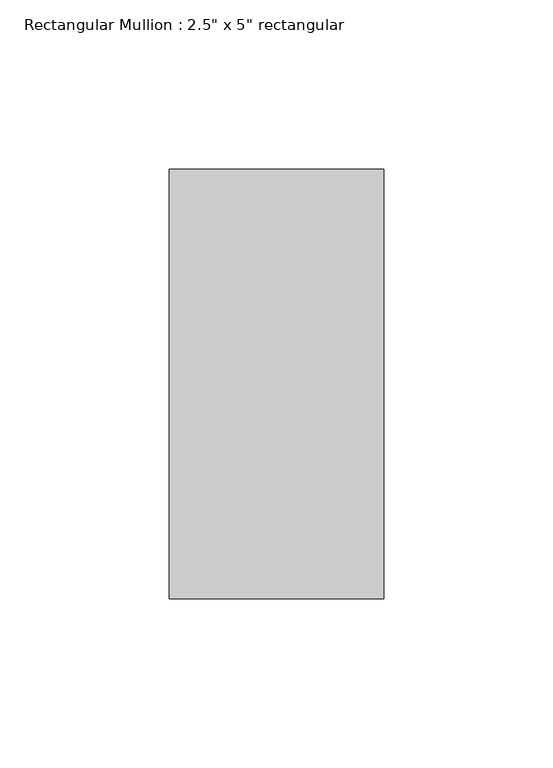
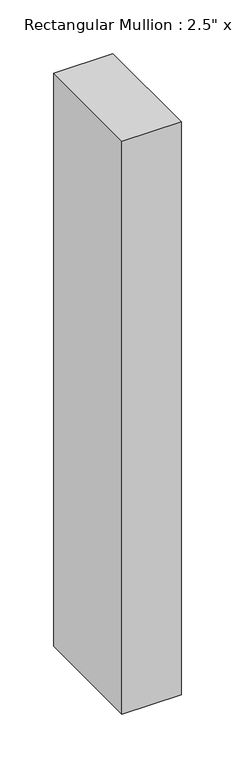
"""IFC4 building model written with IfcOpenShell, lengths in millimetres: member geometry."""

from ifc_helpers import new_model, si_unit, frame, origin, place, context, project, spatial, polyline, outline, extrude, source, transform, mapped, element, save


def member_21c47307(model_context):
    return source(origin(), model_context, "Body", "SweptSolid", [
        extrude(outline(polyline([(0.0, 63.5), (0.0, -63.5), (-63.5, -63.5), (-63.5, 63.5), (0.0, 63.5)])), frame((0.0, 0.0, -651.1147026), z_axis=(0.0, 0.0, 1.0), x_axis=(1.0, 0.0, 0.0)), (0.0, 0.0, 1.0), 651.1147026),
    ])


if __name__ == "__main__":
    model = new_model("IFC4")
    model_context = context("Model", 3, world=origin())
    ifc_project = project(units=[si_unit("LENGTHUNIT", "METRE", prefix="MILLI")], contexts=[model_context])
    site = spatial("IfcSite", under=ifc_project)
    building = spatial("IfcBuilding", under=site)
    placement = place(None, origin())
    member_shape = member_21c47307(model_context)
    element("IfcMember", 1, ObjectType="Rectangular Mullion : 2.5\" x 5\" rectangular", at=placement, inside=building, context=model_context, shape_type="MappedRepresentation", body=[
        mapped(member_shape, transform((0.0, 0.0, 0.0), x_axis=(1.0, 0.0, 0.0), y_axis=(0.0, 1.0, 0.0), z_axis=(0.0, 0.0, 1.0))),
    ])
    save(model, "model.ifc")

# Revit data of these elements
# Type "Rectangular Mullion : 2.5\" x 5\" rectangular"
#   built-in parameter 1007304 = 0.416667 (stored number, unit not read)
#   built-in parameter 1007301 = 0.104167 (stored number, unit not read)
#   built-in parameter 1007300 = 0.104167 (stored number, unit not read)
# Element 1 (IfcMember, "Rectangular Mullion : 2.5\" x 5\" rectangular")
#   Materials on its faces: "Aluminum"
# Materials
#   "Aluminum": class "Metal", colour RGB 247 247 247, transparency 0, Description = "Aluminum 6061", Cost = 0
